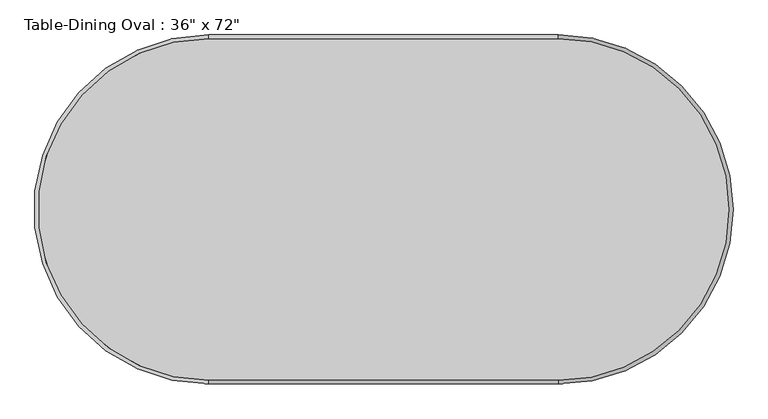
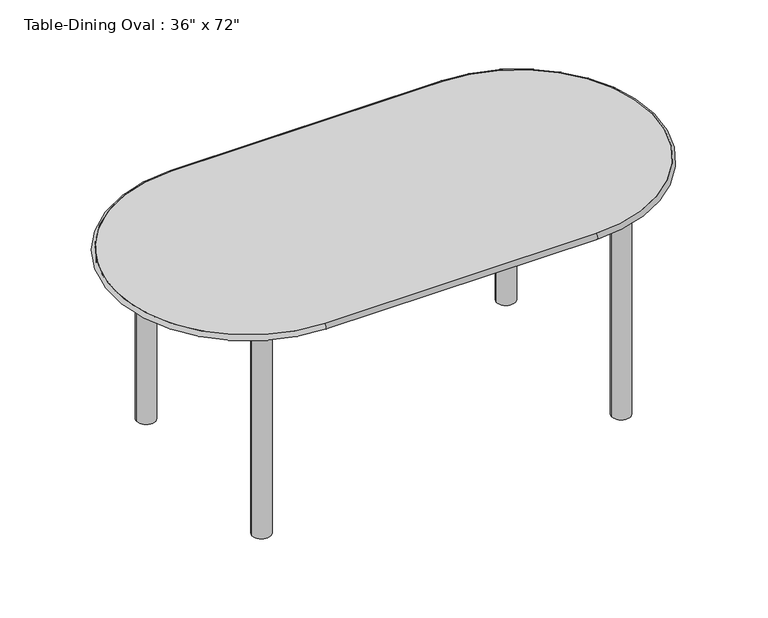
"""IFC4 building model written with IfcOpenShell, lengths in millimetres: furniture geometry."""

from ifc_helpers import new_model, si_unit, point, frame, frame_2d, origin, origin_with_axes, place, context, project, spatial, polyline, circle_curve, ellipse_curve, trimmed, segment, composite_curve, outline, extrude, source, transform, mapped, element, save
from ifc_brep_helpers import plane_surface, cylinder_surface, revolved_surface, advanced_brep


def furniture_2c34a4f9(model_context):
    return source(origin(), model_context, "Body", "SolidModel", [
        advanced_brep(
        [(-859.0196721, -805.7733607, 762.0), (-859.0196721, -805.7733607, 742.95), (55.3803279, -805.7733607, 742.95), (55.3803279, -805.7733607, 762.0), (55.3803279, 89.5766393, 762.0), (55.3803279, 89.5766393, 742.95), (-859.0196721, 89.5766393, 742.95), (-859.0196721, 89.5766393, 762.0)],
        [
            (0, 1, circle_curve(frame((-859.0196721, -805.7733607, 752.475), z_axis=(1.0, 0.0, 0.0), x_axis=(0.0, 1.0, 0.0)), 9.525)),
            (1, 2),
            (2, 3, circle_curve(frame((55.3803279, -805.7733607, 752.475), z_axis=(-1.0, 0.0, 0.0), x_axis=(0.0, 1.0, 0.0)), 9.525)),
            (3, 0),
            (1, 0),
            (3, 2),
            (4, 3, circle_curve(frame((55.3803279, -358.0983607, 762.0), z_axis=(0.0, 0.0, -1.0), x_axis=(0.0, -1.0, 0.0)), 447.675)),
            (2, 5, circle_curve(frame((55.3803279, -358.0983607, 742.95), z_axis=(0.0, 0.0, 1.0), x_axis=(0.0, -1.0, 0.0)), 447.675)),
            (5, 4, circle_curve(frame((55.3803279, 89.5766393, 752.475), z_axis=(1.0, 0.0, 0.0), x_axis=(0.0, -1.0, 0.0)), 9.525)),
            (4, 5),
            (5, 6),
            (6, 7, circle_curve(frame((-859.0196721, 89.5766393, 752.475), z_axis=(1.0, 0.0, 0.0), x_axis=(0.0, -1.0, 0.0)), 9.525)),
            (7, 4),
            (7, 6),
            (0, 7, circle_curve(frame((-859.0196721, -358.0983607, 762.0), z_axis=(0.0, 0.0, -1.0), x_axis=(0.0, 1.0, 0.0)), 447.675)),
            (6, 1, circle_curve(frame((-859.0196721, -358.0983607, 742.95), z_axis=(0.0, 0.0, 1.0), x_axis=(0.0, 1.0, 0.0)), 447.675)),
        ],
        [
            cylinder_surface(frame((-859.0196721, -805.7733607, 752.475), z_axis=(-1.0, 0.0, 0.0), x_axis=(0.0, 1.0, 0.0)), 9.525),
            plane_surface(frame((-859.0196721, -805.7733607, 762.0), z_axis=(0.0, 1.0, 0.0), x_axis=(1.0, 0.0, 0.0))),
            revolved_surface(trimmed(ellipse_curve(frame((55.3803279, -805.7733607, 752.475), z_axis=(-1.0, 0.0, 0.0), x_axis=(0.0, 1.0, 0.0)), 9.525, 9.525), [point((55.3803279, -805.7733607, 742.95))], [point((55.3803279, -805.7733607, 762.0))], True, "CARTESIAN"), (55.3803279, -358.0983607, 0.0), (0.0, 0.0, 1.0)),
            revolved_surface(polyline([(55.3803279, -805.7733607, 762.0), (55.3803279, -805.7733607, 742.95)]), (55.3803279, -358.0983607, 0.0), (0.0, 0.0, 1.0)),
            cylinder_surface(frame((55.3803279, 89.5766393, 752.475), z_axis=(1.0, 0.0, 0.0), x_axis=(0.0, -1.0, 0.0)), 9.525),
            plane_surface(frame((55.3803279, 89.5766393, 762.0), z_axis=(0.0, -1.0, 0.0), x_axis=(-1.0, 0.0, 0.0))),
            revolved_surface(trimmed(ellipse_curve(frame((-859.0196721, 89.5766393, 752.475), z_axis=(1.0, 0.0, 0.0), x_axis=(0.0, -1.0, 0.0)), 9.525, 9.525), [point((-859.0196721, 89.5766393, 742.95))], [point((-859.0196721, 89.5766393, 762.0))], True, "CARTESIAN"), (-859.0196721, -358.0983607, 0.0), (0.0, 0.0, 1.0)),
            revolved_surface(polyline([(-859.0196721, 89.57663930000001, 762.0), (-859.0196721, 89.57663930000001, 742.95)]), (-859.0196721, -358.0983607, 0.0), (0.0, 0.0, 1.0)),
        ],
        [
            (0, [[1, 2, 3, 4]]),
            (1, [[5, -4, 6, -2]]),
            (2, [[7, -3, 8, 9]]),
            (3, [[-8, -6, -7, 10]]),
            (4, [[-9, 11, 12, 13]]),
            (5, [[-10, -13, 14, -11]]),
            (6, [[15, -12, 16, -1]]),
            (7, [[-16, -14, -15, -5]]),
        ],
    ),
        extrude(outline(composite_curve([segment(trimmed(circle_curve(frame_2d((-1008.2446721, -21.5483607)), 31.75), [point((-1039.9946721, -21.5483607))], [point((-976.4946721, -21.5483607))], False, "CARTESIAN"), True, "CONTINUOUS"), segment(trimmed(circle_curve(frame_2d((-1008.2446721, -21.5483607)), 31.75), [point((-976.4946721, -21.5483607))], [point((-1039.9946721, -21.5483607))], False, "CARTESIAN"), True, "CONTINUOUS")], self_intersect=False)), origin_with_axes(), (0.0, 0.0, 1.0), 742.95),
        extrude(outline(composite_curve([segment(trimmed(circle_curve(frame_2d((-1008.2446721, -694.6483607)), 31.75), [point((-1039.9946721, -694.6483607))], [point((-976.4946721, -694.6483607))], False, "CARTESIAN"), True, "CONTINUOUS"), segment(trimmed(circle_curve(frame_2d((-1008.2446721, -694.6483607)), 31.75), [point((-976.4946721, -694.6483607))], [point((-1039.9946721, -694.6483607))], False, "CARTESIAN"), True, "CONTINUOUS")], self_intersect=False)), origin_with_axes(), (0.0, 0.0, 1.0), 742.95),
        extrude(outline(composite_curve([segment(trimmed(circle_curve(frame_2d((204.6053279, -21.5483607)), 31.75), [point((172.8553279, -21.5483607))], [point((236.3553279, -21.5483607))], False, "CARTESIAN"), True, "CONTINUOUS"), segment(trimmed(circle_curve(frame_2d((204.6053279, -21.5483607)), 31.75), [point((236.3553279, -21.5483607))], [point((172.8553279, -21.5483607))], False, "CARTESIAN"), True, "CONTINUOUS")], self_intersect=False)), origin_with_axes(), (0.0, 0.0, 1.0), 742.95),
        extrude(outline(composite_curve([segment(trimmed(circle_curve(frame_2d((204.6053279, -694.6483607)), 31.75), [point((172.8553279, -694.6483607))], [point((236.3553279, -694.6483607))], False, "CARTESIAN"), True, "CONTINUOUS"), segment(trimmed(circle_curve(frame_2d((204.6053279, -694.6483607)), 31.75), [point((236.3553279, -694.6483607))], [point((172.8553279, -694.6483607))], False, "CARTESIAN"), True, "CONTINUOUS")], self_intersect=False)), origin_with_axes(), (0.0, 0.0, 1.0), 742.95),
        extrude(outline(polyline([(223.6553279, -2.4983607), (223.6553279, -713.6983607), (-1027.2946721, -713.6983607), (-1027.2946721, -2.4983607), (223.6553279, -2.4983607)]), holes=[polyline([(204.6053279, -21.5483607), (-1008.2446721, -21.5483607), (-1008.2446721, -694.6483607), (204.6053279, -694.6483607), (204.6053279, -21.5483607)])]), frame((0.0, 0.0, 692.15), z_axis=(0.0, 0.0, 1.0), x_axis=(1.0, 0.0, 0.0)), (0.0, 0.0, 1.0), 50.8),
        extrude(outline(composite_curve([segment(polyline([(-859.0196721, 89.5766393), (55.3803279, 89.5766393)]), True, "CONTINUOUS"), segment(trimmed(circle_curve(frame_2d((55.3803279, -358.0983607)), 447.675), [point((55.3803279, 89.5766393))], [point((503.0553279, -358.0983607))], False, "CARTESIAN"), True, "CONTINUOUS"), segment(trimmed(circle_curve(frame_2d((55.3803279, -358.0983607)), 447.675), [point((503.0553279, -358.0983607))], [point((55.3803279, -805.7733607))], False, "CARTESIAN"), True, "CONTINUOUS"), segment(polyline([(55.3803279, -805.7733607), (-859.0196721, -805.7733607)]), True, "CONTINUOUS"), segment(trimmed(circle_curve(frame_2d((-859.0196721, -358.0983607)), 447.675), [point((-859.0196721, -805.7733607))], [point((-1306.6946721, -358.0983607))], False, "CARTESIAN"), True, "CONTINUOUS"), segment(trimmed(circle_curve(frame_2d((-859.0196721, -358.0983607)), 447.675), [point((-1306.6946721, -358.0983607))], [point((-859.0196721, 89.5766393))], False, "CARTESIAN"), True, "CONTINUOUS")], self_intersect=False)), frame((0.0, 0.0, 742.95), z_axis=(0.0, 0.0, 1.0), x_axis=(1.0, 0.0, 0.0)), (0.0, 0.0, 1.0), 19.05),
    ])


if __name__ == "__main__":
    model = new_model("IFC4")
    model_context = context("Model", 3, world=origin())
    ifc_project = project(units=[si_unit("LENGTHUNIT", "METRE", prefix="MILLI")], contexts=[model_context])
    site = spatial("IfcSite", under=ifc_project)
    building = spatial("IfcBuilding", under=site)
    placement = place(None, origin())
    furniture_shape = furniture_2c34a4f9(model_context)
    element("IfcFurniture", 1, ObjectType="Table-Dining Oval : 36\" x 72\"", at=placement, inside=building, context=model_context, shape_type="MappedRepresentation", body=[
        mapped(furniture_shape, transform((0.0, 0.0, 0.0), x_axis=(1.0, 0.0, 0.0), y_axis=(0.0, 1.0, 0.0), z_axis=(0.0, 0.0, 1.0))),
    ])
    save(model, "model.ifc")

# Revit data of these elements
# Type "Table-Dining Oval : 36\" x 72\""
#   Assembly Code = "E2020200"
#   Length = 6' - 0"
#   Width = 3' - 0"
#   Base Material = Steel, Chrome Plated
#   Top Material = Glass - Clear, Grey
#   Description = (empty or 0)
# Element 1 (IfcFurniture, "Table-Dining Oval : 36\" x 72\"")
#   Materials on its faces: "Steel, Chrome Plated", "Glass - Clear, Grey"
# Materials
#   "Steel, Chrome Plated": class "Metal", colour RGB 17 17 17, transparency 0, Description = "Chromiuim plated steel", Cost = 0
#   "Glass - Clear, Grey": class "Glass", colour RGB 252 255 255, transparency 0.64
